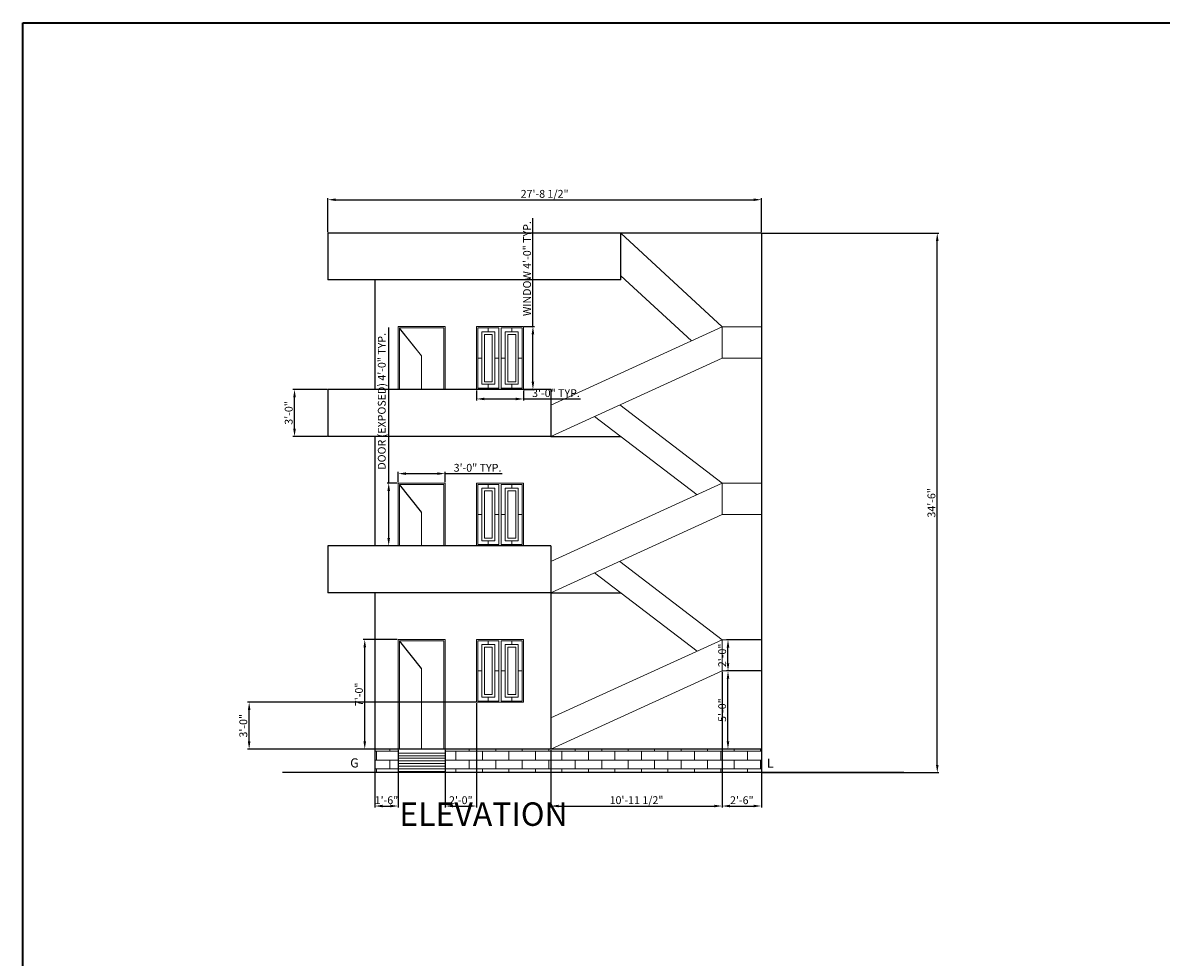
# Model space of a CAD drawing. Units: millimetres. Extents: x 50579 to 52843, y 62224 to 63803.
# Tile 2 of 5: x 50579 to 51453, y 63086 to 63803. Entities that reach past the tile are written whole.
import ezdxf

# ---------------------------------------------------------------- set-up
doc = ezdxf.new("R2010")
doc.units = ezdxf.units.MM
for name, color, linetype, lineweight in [('A-ANNO-DIMS', 2, 'Continuous', 18), ('A-ANNO-SYMB', 6, 'Continuous', 18), ('A-ANNO-TITL', 4, 'Continuous', 25), ('A-ANNO-TTLB', 7, 'Continuous', 35), ('A-ELEV', 7, 'Continuous', 25), ('A-ELEV-OPEN', 7, 'Continuous', 18), ('A-ELEV-PATT', 8, 'Continuous', 13), ('A-ELEV-STRS', 7, 'Continuous', 18)]:
    doc.layers.add(name, color=color, linetype=linetype, lineweight=lineweight)
doc.styles.get("Standard").update_dxf_attribs({"font": 'arial.ttf'})
doc.dimstyles.new('ISO-25', dxfattribs={"dimtxt": 6, "dimasz": 6, "dimexe": 1.25, "dimexo": 0.625, "dimtad": 1, "dimdec": 0, "dimlunit": 3, "dimtxsty": 'Standard', "dimcen": 2.5, "dimadec": 0, "dimazin": 0, "dimtfac": 1, "dimtdec": 0, "dimtmove": 0, "dimatfit": 3, "dimfxl": 1, "dimarcsym": 0})

# ---------------------------------------------------------------- blocks, each defined once
blk = doc.blocks.new('DOOR-BALCONY-ELEV')
for p, q in [((36, 48.21), (0, 48.21)), ((0, 48.21), (0, 0)), ((35, 47.21), (1, 47.21)), ((1, 47.21), (1, 0)), ((1, 47.12), (18.01, 25.89)), ((1, 46.8), (17.9, 25.71)), ((35, 0), (35, 47.21)), ((36, 0), (36, 48.21)), ((17.9, 25.71), (17.9, 0)), ((18.01, 25.89), (18.01, 0)), ((0, 0), (36, 0))]:
    blk.add_line(p, q)
blk = doc.blocks.new('WIN-PAIRED-ELEV')
for p, q in [((9, 44.24), (9, 47.24)), ((14, 44.24), (14, 4)), ((17, 47.24), (17, 1)), ((19, 47.24), (19, 1)), ((22, 44.24), (22, 4)), ((27, 44.24), (27, 47.24)), ((4, 24.12), (1, 24.12)), ((17, 24.12), (14, 24.12)), ((19, 24.12), (22, 24.12)), ((32, 24.12), (35, 24.12)), ((9, 4), (9, 1)), ((27, 4), (27, 1))]:
    blk.add_line(p, q)
for points in [[(0, 48.24), (36, 48.24), (36, 0), (0, 0)], [(12, 6), (6, 6), (6, 42.24), (12, 42.24)], [(24, 42.24), (30, 42.24), (30, 6), (24, 6)]]:
    blk.add_lwpolyline(points, close=True)
for points in [[(17, 1), (1, 1), (1, 47.24), (17, 47.24)], [(14, 4), (4, 4), (4, 44.24), (14, 44.24)], [(19, 47.24), (35, 47.24), (35, 1), (19, 1)], [(22, 44.24), (32, 44.24), (32, 4), (22, 4)]]:
    blk.add_lwpolyline(points)
blk = doc.blocks.new('*D37')
at = {"layer": 'A-ANNO-DIMS', "color": 0, "lineweight": -2, "transparency": 16777216}
for p, q in [((50860.17, 63449.49), (50860.17, 63568.92)), ((50866.77, 63449.49), (50858.92, 63449.49)), ((50860.17, 63407.28), (50860.17, 63443.49)), ((50866.77, 63401.28), (50858.92, 63401.28))]:
    blk.add_line(p, q, dxfattribs=at)
at = {"layer": 'A-ANNO-DIMS', "color": 0, "transparency": 16777216}
for points in [[(50859.17, 63443.49), (50861.17, 63443.49), (50860.17, 63449.49)], [(50859.17, 63407.28), (50861.17, 63407.28), (50860.17, 63401.28)]]:
    blk.add_solid(points, dxfattribs=at)
at = {"layer": 'Defpoints', "color": 0, "transparency": 16777216}
for p in [(50860.17, 63449.49), (50867.4, 63449.49), (50867.4, 63401.28)]:
    blk.add_point(p, dxfattribs=at)
at = {"layer": 'A-ANNO-DIMS', "color": 0, "transparency": 16777216, "insert": (50855.61, 63512.2), "char_height": 6, "attachment_point": 5, "rotation": 90}
blk.add_mtext('DOOR (EXPOSED) 4\'-0" TYP.', dxfattribs=at)
blk = doc.blocks.new('*D38')
at = {"layer": 'A-ANNO-DIMS', "color": 0, "lineweight": -2, "transparency": 16777216}
for p, q in [((50867.4, 63450.11), (50867.4, 63457.97)), ((50873.4, 63456.72), (50897.4, 63456.72)), ((50903.4, 63450.11), (50903.4, 63457.97)), ((50903.4, 63456.72), (50947.22, 63456.72))]:
    blk.add_line(p, q, dxfattribs=at)
at = {"layer": 'A-ANNO-DIMS', "color": 0, "transparency": 16777216}
for points in [[(50873.4, 63457.72), (50873.4, 63455.72), (50867.4, 63456.72)], [(50897.4, 63457.72), (50897.4, 63455.72), (50903.4, 63456.72)]]:
    blk.add_solid(points, dxfattribs=at)
at = {"layer": 'Defpoints', "color": 0, "transparency": 16777216}
for p in [(50903.4, 63456.72), (50867.4, 63449.49), (50903.4, 63449.49)]:
    blk.add_point(p, dxfattribs=at)
at = {"layer": 'A-ANNO-DIMS', "color": 0, "transparency": 16777216, "insert": (50928.31, 63460.41), "char_height": 6, "attachment_point": 5}
blk.add_mtext('3\'-0" TYP.', dxfattribs=at)
blk = doc.blocks.new('*D39')
at = {"layer": 'A-ANNO-DIMS', "color": 0, "lineweight": -2, "transparency": 16777216}
for p, q in [((50970.79, 63569.49), (50970.79, 63652.66)), ((50964.18, 63569.49), (50972.04, 63569.49)), ((50970.79, 63527.25), (50970.79, 63563.49)), ((50964.18, 63521.25), (50972.04, 63521.25))]:
    blk.add_line(p, q, dxfattribs=at)
at = {"layer": 'A-ANNO-DIMS', "color": 0, "transparency": 16777216}
for points in [[(50969.79, 63563.49), (50971.79, 63563.49), (50970.79, 63569.49)], [(50969.79, 63527.25), (50971.79, 63527.25), (50970.79, 63521.25)]]:
    blk.add_solid(points, dxfattribs=at)
at = {"layer": 'Defpoints', "color": 0, "transparency": 16777216}
for p in [(50963.56, 63569.49), (50970.79, 63569.49), (50963.56, 63521.25)]:
    blk.add_point(p, dxfattribs=at)
at = {"layer": 'A-ANNO-DIMS', "color": 0, "transparency": 16777216, "insert": (50967.06, 63614.07), "char_height": 6, "attachment_point": 5, "rotation": 90}
blk.add_mtext('WINDOW 4\'-0" TYP.', dxfattribs=at)
blk = doc.blocks.new('*D40')
at = {"layer": 'A-ANNO-DIMS', "color": 0, "lineweight": -2, "transparency": 16777216}
for p, q in [((50927.56, 63520.62), (50927.56, 63512.76)), ((50963.56, 63520.62), (50963.56, 63512.76)), ((50933.56, 63514.01), (50957.56, 63514.01)), ((50963.56, 63514.01), (51007.37, 63514.01))]:
    blk.add_line(p, q, dxfattribs=at)
at = {"layer": 'A-ANNO-DIMS', "color": 0, "transparency": 16777216}
for points in [[(50933.56, 63515.01), (50933.56, 63513.01), (50927.56, 63514.01)], [(50957.56, 63515.01), (50957.56, 63513.01), (50963.56, 63514.01)]]:
    blk.add_solid(points, dxfattribs=at)
at = {"layer": 'Defpoints', "color": 0, "transparency": 16777216}
for p in [(50927.56, 63521.25), (50963.56, 63521.25), (50963.56, 63514.01)]:
    blk.add_point(p, dxfattribs=at)
at = {"layer": 'A-ANNO-DIMS', "color": 0, "transparency": 16777216, "insert": (50988.47, 63517.7), "char_height": 6, "attachment_point": 5}
blk.add_mtext('3\'-0" TYP.', dxfattribs=at)
blk = doc.blocks.new('*D45')
at = {"layer": 'A-ANNO-DIMS', "color": 0, "lineweight": -2, "transparency": 16777216}
for p, q in [((50813.52, 63641.9), (50813.52, 63668.13)), ((50819.52, 63666.88), (51140.02, 63666.88)), ((51146.02, 63641.9), (51146.02, 63668.13))]:
    blk.add_line(p, q, dxfattribs=at)
at = {"layer": 'A-ANNO-DIMS', "color": 0, "transparency": 16777216}
for points in [[(50819.52, 63667.88), (50819.52, 63665.88), (50813.52, 63666.88)], [(51140.02, 63667.88), (51140.02, 63665.88), (51146.02, 63666.88)]]:
    blk.add_solid(points, dxfattribs=at)
at = {"layer": 'Defpoints', "color": 0, "transparency": 16777216}
for p in [(51146.02, 63666.88), (50813.52, 63641.28), (51146.02, 63641.28)]:
    blk.add_point(p, dxfattribs=at)
at = {"layer": 'A-ANNO-DIMS', "color": 0, "transparency": 16777216, "insert": (50979.77, 63670.61), "char_height": 6, "attachment_point": 5}
blk.add_mtext('27\'-8 1/2"', dxfattribs=at)
blk = doc.blocks.new('*D46')
at = {"layer": 'A-ANNO-DIMS', "color": 0, "lineweight": -2, "transparency": 16777216}
for p, q in [((51146.64, 63641.28), (51282.2, 63641.28)), ((51280.95, 63233.28), (51280.95, 63635.28)), ((51146.64, 63227.28), (51282.2, 63227.28))]:
    blk.add_line(p, q, dxfattribs=at)
at = {"layer": 'A-ANNO-DIMS', "color": 0, "transparency": 16777216}
for points in [[(51279.95, 63635.28), (51281.95, 63635.28), (51280.95, 63641.28)], [(51279.95, 63233.28), (51281.95, 63233.28), (51280.95, 63227.28)]]:
    blk.add_solid(points, dxfattribs=at)
at = {"layer": 'Defpoints', "color": 0, "transparency": 16777216}
for p in [(51146.02, 63641.28), (51280.95, 63641.28), (51146.02, 63227.28)]:
    blk.add_point(p, dxfattribs=at)
at = {"layer": 'A-ANNO-DIMS', "color": 0, "transparency": 16777216, "insert": (51277.26, 63434.28), "char_height": 6, "attachment_point": 5, "rotation": 90}
blk.add_mtext('34\'-6"', dxfattribs=at)
blk = doc.blocks.new('*D49')
at = {"layer": 'A-ANNO-DIMS', "color": 0, "lineweight": -2, "transparency": 16777216}
for p, q in [((50849.52, 63244.65), (50849.52, 63200.43)), ((50867.4, 63244.65), (50867.4, 63200.43)), ((50855.52, 63201.68), (50861.4, 63201.68))]:
    blk.add_line(p, q, dxfattribs=at)
at = {"layer": 'A-ANNO-DIMS', "color": 0, "transparency": 16777216}
for points in [[(50855.52, 63202.68), (50855.52, 63200.68), (50849.52, 63201.68)], [(50861.4, 63202.68), (50861.4, 63200.68), (50867.4, 63201.68)]]:
    blk.add_solid(points, dxfattribs=at)
at = {"layer": 'Defpoints', "color": 0, "transparency": 16777216}
for p in [(50849.52, 63245.28), (50867.4, 63245.28), (50867.4, 63201.68)]:
    blk.add_point(p, dxfattribs=at)
at = {"layer": 'A-ANNO-DIMS', "color": 0, "transparency": 16777216, "insert": (50858.46, 63205.37), "char_height": 6, "attachment_point": 5}
blk.add_mtext('1\'-6"', dxfattribs=at)
blk = doc.blocks.new('*D50')
at = {"layer": 'A-ANNO-DIMS', "color": 0, "lineweight": -2, "transparency": 16777216}
for p, q in [((50927.56, 63280.62), (50927.56, 63200.43)), ((50903.4, 63244.65), (50903.4, 63200.43)), ((50909.4, 63201.68), (50921.56, 63201.68))]:
    blk.add_line(p, q, dxfattribs=at)
at = {"layer": 'A-ANNO-DIMS', "color": 0, "transparency": 16777216}
for points in [[(50909.4, 63202.68), (50909.4, 63200.68), (50903.4, 63201.68)], [(50921.56, 63202.68), (50921.56, 63200.68), (50927.56, 63201.68)]]:
    blk.add_solid(points, dxfattribs=at)
at = {"layer": 'Defpoints', "color": 0, "transparency": 16777216}
for p in [(50927.56, 63281.25), (50903.4, 63245.28), (50927.56, 63201.68)]:
    blk.add_point(p, dxfattribs=at)
at = {"layer": 'A-ANNO-DIMS', "color": 0, "transparency": 16777216, "insert": (50915.48, 63205.37), "char_height": 6, "attachment_point": 5}
blk.add_mtext('2\'-0"', dxfattribs=at)
blk = doc.blocks.new('*D51')
at = {"layer": 'A-ANNO-DIMS', "color": 0, "lineweight": -2, "transparency": 16777216}
for p, q in [((51116.02, 63304.65), (51116.02, 63200.43)), ((50984.52, 63244.65), (50984.52, 63200.43)), ((50990.52, 63201.68), (51110.02, 63201.68))]:
    blk.add_line(p, q, dxfattribs=at)
at = {"layer": 'A-ANNO-DIMS', "color": 0, "transparency": 16777216}
for points in [[(50990.52, 63202.68), (50990.52, 63200.68), (50984.52, 63201.68)], [(51110.02, 63202.68), (51110.02, 63200.68), (51116.02, 63201.68)]]:
    blk.add_solid(points, dxfattribs=at)
at = {"layer": 'Defpoints', "color": 0, "transparency": 16777216}
for p in [(51116.02, 63305.28), (50984.52, 63245.28), (51116.02, 63201.68)]:
    blk.add_point(p, dxfattribs=at)
at = {"layer": 'A-ANNO-DIMS', "color": 0, "transparency": 16777216, "insert": (51050.27, 63205.41), "char_height": 6, "attachment_point": 5}
blk.add_mtext('10\'-11 1/2"', dxfattribs=at)
blk = doc.blocks.new('*D52')
at = {"layer": 'A-ANNO-DIMS', "color": 0, "lineweight": -2, "transparency": 16777216}
for p, q in [((51116.02, 63304.65), (51116.02, 63200.43)), ((51146.02, 63244.65), (51146.02, 63200.43)), ((51122.02, 63201.68), (51140.02, 63201.68))]:
    blk.add_line(p, q, dxfattribs=at)
at = {"layer": 'A-ANNO-DIMS', "color": 0, "transparency": 16777216}
for points in [[(51122.02, 63202.68), (51122.02, 63200.68), (51116.02, 63201.68)], [(51140.02, 63202.68), (51140.02, 63200.68), (51146.02, 63201.68)]]:
    blk.add_solid(points, dxfattribs=at)
at = {"layer": 'Defpoints', "color": 0, "transparency": 16777216}
for p in [(51116.02, 63305.28), (51146.02, 63245.28), (51146.02, 63201.68)]:
    blk.add_point(p, dxfattribs=at)
at = {"layer": 'A-ANNO-DIMS', "color": 0, "transparency": 16777216, "insert": (51131.02, 63205.37), "char_height": 6, "attachment_point": 5}
blk.add_mtext('2\'-6"', dxfattribs=at)
blk = doc.blocks.new('*D53')
at = {"layer": 'A-ANNO-DIMS', "color": 0, "lineweight": -2, "transparency": 16777216}
for p, q in [((50926.93, 63281.25), (50751.87, 63281.25)), ((50753.12, 63251.28), (50753.12, 63275.25)), ((50866.77, 63245.28), (50751.87, 63245.28))]:
    blk.add_line(p, q, dxfattribs=at)
at = {"layer": 'A-ANNO-DIMS', "color": 0, "transparency": 16777216}
for points in [[(50752.12, 63275.25), (50754.12, 63275.25), (50753.12, 63281.25)], [(50752.12, 63251.28), (50754.12, 63251.28), (50753.12, 63245.28)]]:
    blk.add_solid(points, dxfattribs=at)
at = {"layer": 'Defpoints', "color": 0, "transparency": 16777216}
for p in [(50753.12, 63281.25), (50927.56, 63281.25), (50867.4, 63245.28)]:
    blk.add_point(p, dxfattribs=at)
at = {"layer": 'A-ANNO-DIMS', "color": 0, "transparency": 16777216, "insert": (50749.42, 63263.26), "char_height": 6, "attachment_point": 5, "rotation": 90}
blk.add_mtext('3\'-0"', dxfattribs=at)
blk = doc.blocks.new('*D54')
at = {"layer": 'A-ANNO-DIMS', "color": 0, "lineweight": -2, "transparency": 16777216}
for p, q in [((50866.77, 63329.49), (50840.55, 63329.49)), ((50841.8, 63251.28), (50841.8, 63323.49)), ((50866.77, 63245.28), (50840.55, 63245.28))]:
    blk.add_line(p, q, dxfattribs=at)
at = {"layer": 'A-ANNO-DIMS', "color": 0, "transparency": 16777216}
for points in [[(50840.8, 63323.49), (50842.8, 63323.49), (50841.8, 63329.49)], [(50840.8, 63251.28), (50842.8, 63251.28), (50841.8, 63245.28)]]:
    blk.add_solid(points, dxfattribs=at)
at = {"layer": 'Defpoints', "color": 0, "transparency": 16777216}
for p in [(50841.8, 63329.49), (50867.4, 63329.49), (50867.4, 63245.28)]:
    blk.add_point(p, dxfattribs=at)
at = {"layer": 'A-ANNO-DIMS', "color": 0, "transparency": 16777216, "insert": (50838.11, 63287.38), "char_height": 6, "attachment_point": 5, "rotation": 90}
blk.add_mtext('7\'-0"', dxfattribs=at)
blk = doc.blocks.new('*D55')
at = {"layer": 'A-ANNO-DIMS', "color": 0, "lineweight": -2, "transparency": 16777216}
for p, q in [((51145.39, 63305.28), (51119.17, 63305.28)), ((51120.42, 63251.28), (51120.42, 63299.28)), ((51145.39, 63245.28), (51119.17, 63245.28))]:
    blk.add_line(p, q, dxfattribs=at)
at = {"layer": 'A-ANNO-DIMS', "color": 0, "transparency": 16777216}
for points in [[(51119.42, 63299.28), (51121.42, 63299.28), (51120.42, 63305.28)], [(51119.42, 63251.28), (51121.42, 63251.28), (51120.42, 63245.28)]]:
    blk.add_solid(points, dxfattribs=at)
at = {"layer": 'Defpoints', "color": 0, "transparency": 16777216}
for p in [(51120.42, 63305.28), (51146.02, 63305.28), (51146.02, 63245.28)]:
    blk.add_point(p, dxfattribs=at)
at = {"layer": 'A-ANNO-DIMS', "color": 0, "transparency": 16777216, "insert": (51116.73, 63275.28), "char_height": 6, "attachment_point": 5, "rotation": 90}
blk.add_mtext('5\'-0"', dxfattribs=at)
blk = doc.blocks.new('*D56')
at = {"layer": 'A-ANNO-DIMS', "color": 0, "lineweight": -2, "transparency": 16777216}
for p, q in [((51145.39, 63329.28), (51119.17, 63329.28)), ((51120.42, 63311.28), (51120.42, 63323.28)), ((51145.39, 63305.28), (51119.17, 63305.28))]:
    blk.add_line(p, q, dxfattribs=at)
at = {"layer": 'A-ANNO-DIMS', "color": 0, "transparency": 16777216}
for points in [[(51119.42, 63323.28), (51121.42, 63323.28), (51120.42, 63329.28)], [(51119.42, 63311.28), (51121.42, 63311.28), (51120.42, 63305.28)]]:
    blk.add_solid(points, dxfattribs=at)
at = {"layer": 'Defpoints', "color": 0, "transparency": 16777216}
for p in [(51120.42, 63329.28), (51146.02, 63329.28), (51146.02, 63305.28)]:
    blk.add_point(p, dxfattribs=at)
at = {"layer": 'A-ANNO-DIMS', "color": 0, "transparency": 16777216, "insert": (51116.73, 63317.28), "char_height": 6, "attachment_point": 5, "rotation": 90}
blk.add_mtext('2\'-0"', dxfattribs=at)
blk = doc.blocks.new('*D57')
at = {"layer": 'A-ANNO-DIMS', "color": 0, "lineweight": -2, "transparency": 16777216}
for p, q in [((50812.89, 63521.28), (50786.67, 63521.28)), ((50787.92, 63491.28), (50787.92, 63515.28)), ((50812.89, 63485.28), (50786.67, 63485.28))]:
    blk.add_line(p, q, dxfattribs=at)
at = {"layer": 'A-ANNO-DIMS', "color": 0, "transparency": 16777216}
for points in [[(50786.92, 63515.28), (50788.92, 63515.28), (50787.92, 63521.28)], [(50786.92, 63491.28), (50788.92, 63491.28), (50787.92, 63485.28)]]:
    blk.add_solid(points, dxfattribs=at)
at = {"layer": 'Defpoints', "color": 0, "transparency": 16777216}
for p in [(50787.92, 63521.28), (50813.52, 63521.28), (50813.52, 63485.28)]:
    blk.add_point(p, dxfattribs=at)
at = {"layer": 'A-ANNO-DIMS', "color": 0, "transparency": 16777216, "insert": (50784.23, 63503.28), "char_height": 6, "attachment_point": 5, "rotation": 90}
blk.add_mtext('3\'-0"', dxfattribs=at)

msp = doc.modelspace()

# ---------------------------------------------------------------- hatches: boundary and pattern name
at = {"layer": 'A-ELEV-PATT'}
h = msp.add_hatch(dxfattribs=at)
h.set_pattern_fill('AR-BRSTD', color=256, scale=0.1)
h.paths.add_polyline_path([(50867.4, 63245.28), (50849.52, 63245.28), (50849.52, 63227.28), (50867.4, 63227.28)])
h = msp.add_hatch(dxfattribs=at)
h.set_pattern_fill('AR-BRSTD', color=256, scale=0.1)
h.paths.add_polyline_path([(51146.02, 63245.28), (50903.4, 63245.28), (50903.4, 63227.28), (51146.02, 63227.28)])

# ---------------------------------------------------------------- linework, layer by layer
at = {"layer": 'A-ANNO-TTLB'}
msp.add_lwpolyline([(50579.46, 63802.65), (52843.1, 63802.65), (52843.1, 62224.04), (50579.46, 62224.04)], close=True, dxfattribs=at)
at = {"layer": 'A-ELEV'}
for p, q in [((51146.02, 63641.28), (50813.52, 63641.28)), ((50813.52, 63641.28), (50813.52, 63605.28)), ((51038.17, 63605.28), (51038.17, 63641.28)), ((51146.02, 63641.28), (51146.02, 63227.28)), ((51038.17, 63605.28), (50813.52, 63605.28)), ((50849.52, 63605.28), (50849.52, 63521.28)), ((50984.52, 63521.28), (50813.52, 63521.28)), ((50813.52, 63521.28), (50813.52, 63485.28)), ((50984.52, 63521.28), (50984.52, 63485.28)), ((50984.52, 63485.28), (50813.52, 63485.28)), ((50849.52, 63485.28), (50849.52, 63401.28)), ((50984.52, 63485.28), (51038.17, 63485.28)), ((50813.52, 63401.28), (50813.52, 63365.28)), ((50984.52, 63401.28), (50813.52, 63401.28)), ((50984.52, 63401.28), (50984.52, 63245.28)), ((50984.52, 63365.28), (50813.52, 63365.28)), ((50849.52, 63365.28), (50849.52, 63227.28)), ((50984.52, 63365.28), (51038.17, 63365.28)), ((51146.02, 63245.28), (50849.52, 63245.28)), ((51255.35, 63227.28), (50778.72, 63227.28))]:
    msp.add_line(p, q, dxfattribs=at)
at = {"layer": 'A-ELEV-OPEN'}
for p, q in [((50868.4, 63328.4), (50885.41, 63307.17)), ((50868.4, 63328.08), (50885.3, 63306.99)), ((50936.56, 63325.49), (50936.56, 63328.49)), ((50944.56, 63328.49), (50944.56, 63282.25)), ((50946.56, 63328.49), (50946.56, 63282.25)), ((50954.56, 63325.49), (50954.56, 63328.49)), ((50885.3, 63306.99), (50885.3, 63245.28)), ((50885.41, 63307.17), (50885.41, 63245.28)), ((50931.56, 63305.37), (50928.56, 63305.37)), ((50944.56, 63305.37), (50941.56, 63305.37)), ((50946.56, 63305.37), (50949.56, 63305.37)), ((50959.56, 63305.37), (50962.56, 63305.37)), ((50936.56, 63285.25), (50936.56, 63282.25)), ((50954.56, 63285.25), (50954.56, 63282.25))]:
    msp.add_line(p, q, dxfattribs=at)
for points in [[(50867.4, 63245.28), (50903.4, 63245.28), (50903.4, 63329.49), (50867.4, 63329.49)], [(50927.56, 63329.49), (50963.56, 63329.49), (50963.56, 63281.25), (50927.56, 63281.25)], [(50941.56, 63285.25), (50931.56, 63285.25), (50931.56, 63325.49), (50941.56, 63325.49)], [(50939.56, 63287.25), (50933.56, 63287.25), (50933.56, 63323.49), (50939.56, 63323.49)], [(50949.56, 63325.49), (50959.56, 63325.49), (50959.56, 63285.25), (50949.56, 63285.25)], [(50951.56, 63323.49), (50957.56, 63323.49), (50957.56, 63287.25), (50951.56, 63287.25)]]:
    msp.add_lwpolyline(points, close=True, dxfattribs=at)
for points in [[(50902.4, 63245.28), (50902.4, 63328.49), (50868.4, 63328.49), (50868.4, 63245.28)], [(50944.56, 63282.25), (50928.56, 63282.25), (50928.56, 63328.49), (50944.56, 63328.49)], [(50946.56, 63328.49), (50962.56, 63328.49), (50962.56, 63282.25), (50946.56, 63282.25)], [(50885.3, 63246.28), (50885.41, 63246.28)]]:
    msp.add_lwpolyline(points, dxfattribs=at)
at = {"layer": 'A-ELEV-STRS'}
for p, q in [((51038.17, 63641.28), (51116.02, 63569.28)), ((51038.17, 63608.59), (51092.35, 63558.48)), ((50984.52, 63509.28), (51116.02, 63569.28)), ((51116.02, 63569.28), (51116.02, 63545.28)), ((51146.02, 63569.28), (51116.02, 63569.28)), ((50984.52, 63485.28), (51116.02, 63545.28)), ((51146.02, 63545.28), (51116.02, 63545.28)), ((51116.02, 63449.28), (51037.38, 63509.4)), ((51096.75, 63440.49), (51018.12, 63500.61)), ((50984.52, 63389.28), (51116.02, 63449.28)), ((51146.02, 63449.28), (51116.02, 63449.28)), ((51116.02, 63449.28), (51116.02, 63425.28)), ((50984.52, 63365.28), (51116.02, 63425.28)), ((51146.02, 63425.28), (51116.02, 63425.28)), ((51116.02, 63329.28), (51037.38, 63389.4)), ((51096.75, 63320.49), (51018.12, 63380.61)), ((50984.52, 63269.28), (51116.02, 63329.28)), ((51146.02, 63329.28), (51116.02, 63329.28)), ((51116.02, 63329.28), (51116.02, 63305.28)), ((50984.52, 63245.28), (51116.02, 63305.28)), ((51146.02, 63305.28), (51116.02, 63305.28)), ((50867.4, 63245.28), (50867.4, 63227.28)), ((50903.4, 63245.28), (50903.4, 63227.28)), ((50867.4, 63242.28), (50903.4, 63242.28)), ((50867.4, 63240.28), (50903.4, 63240.28)), ((50867.4, 63238.28), (50903.4, 63238.28)), ((50867.4, 63236.28), (50903.4, 63236.28)), ((50867.4, 63234.28), (50903.4, 63234.28)), ((50867.4, 63232.28), (50903.4, 63232.28)), ((50867.4, 63230.28), (50903.4, 63230.28)), ((50867.4, 63228.28), (50903.4, 63228.28))]:
    msp.add_line(p, q, dxfattribs=at)

# ---------------------------------------------------------------- block references
at = {"layer": 'A-ELEV-OPEN'}
for name, p in [('DOOR-BALCONY-ELEV', (50867.4, 63521.28)), ('WIN-PAIRED-ELEV', (50927.56, 63521.25)), ('DOOR-BALCONY-ELEV', (50867.4, 63401.28)), ('WIN-PAIRED-ELEV', (50927.56, 63401.25))]:
    msp.add_blockref(name, p, dxfattribs=at)

# ---------------------------------------------------------------- texts
at = {"layer": 'A-ANNO-SYMB', "char_height": 7, "attachment_point": 1}
for s, insert in [('  G', (50826.33, 63238.26)), ('  L', (51145.99, 63238.04))]:
    msp.add_mtext_dynamic_manual_height_columns(s, width=13.8936, gutter_width=12.5, heights=[0], dxfattribs=dict(at, insert=insert))
at = {"layer": 'A-ANNO-TITL', "insert": (50857.28, 63204.47), "char_height": 18, "attachment_point": 1}
msp.add_mtext_dynamic_manual_height_columns('  ELEVATION', width=341.9217, gutter_width=12.5, heights=[0], dxfattribs=at)

# ---------------------------------------------------------------- dimensions: what is measured, and where the dimension line sits
at = {"layer": 'A-ANNO-DIMS'}
for base, p1, p2, picture, middle in [((51146.02, 63666.88), (50813.52, 63641.28), (51146.02, 63641.28), '*D45', (50979.77, 63670.61)), ((51116.02, 63201.68), (50984.52, 63245.28), (51116.02, 63305.28), '*D51', (51050.27, 63205.41)), ((51146.02, 63201.68), (51116.02, 63305.28), (51146.02, 63245.28), '*D52', (51131.02, 63205.37)), ((50927.56, 63201.68), (50903.4, 63245.28), (50927.56, 63281.25), '*D50', (50915.48, 63205.37)), ((50867.4, 63201.68), (50849.52, 63245.28), (50867.4, 63245.28), '*D49', (50858.46, 63205.37))]:
    dim = msp.add_linear_dim(base=base, p1=p1, p2=p2, dimstyle='ISO-25', override={"dimdec": 1, "dimlfac": 1, "dimrnd": 0, "dimzin": 1, "dimdsep": 46, "dimlunit": 4, "dimfrac": 2}, dxfattribs=at)
    dim.commit()
    dim.dimension.update_dxf_attribs({"geometry": picture, "text_midpoint": middle})
for base, p1, p2, text, picture, middle in [((50970.79, 63569.49), (50963.56, 63521.25), (50963.56, 63569.49), 'WINDOW <> TYP.', '*D39', (50967.06, 63614.07)), ((50860.17, 63449.49), (50867.4, 63401.28), (50867.4, 63449.49), 'DOOR (EXPOSED) <> TYP.', '*D37', (50855.61, 63512.2))]:
    dim = msp.add_linear_dim(base=base, p1=p1, p2=p2, angle=90, text=text, dimstyle='ISO-25', override={"dimdec": 1, "dimlfac": 1, "dimrnd": 0, "dimzin": 1, "dimdsep": 46, "dimlunit": 4, "dimfrac": 2}, dxfattribs=at)
    dim.commit()
    dim.dimension.update_dxf_attribs({"geometry": picture, "text_midpoint": middle})
for base, p1, p2, picture, middle in [((51280.95, 63641.28), (51146.02, 63227.28), (51146.02, 63641.28), '*D46', (51277.26, 63434.28)), ((50787.92, 63521.28), (50813.52, 63485.28), (50813.52, 63521.28), '*D57', (50784.23, 63503.28)), ((50841.8, 63329.49), (50867.4, 63245.28), (50867.4, 63329.49), '*D54', (50838.11, 63287.38)), ((51120.42, 63329.28), (51146.02, 63305.28), (51146.02, 63329.28), '*D56', (51116.73, 63317.28)), ((51120.42, 63305.28), (51146.02, 63245.28), (51146.02, 63305.28), '*D55', (51116.73, 63275.28)), ((50753.12, 63281.25), (50867.4, 63245.28), (50927.56, 63281.25), '*D53', (50749.42, 63263.26))]:
    dim = msp.add_linear_dim(base=base, p1=p1, p2=p2, angle=90, dimstyle='ISO-25', override={"dimdec": 1, "dimlfac": 1, "dimrnd": 0, "dimzin": 1, "dimdsep": 46, "dimlunit": 4, "dimfrac": 2}, dxfattribs=at)
    dim.commit()
    dim.dimension.update_dxf_attribs({"geometry": picture, "text_midpoint": middle})
for base, p1, p2, picture, middle in [((50963.56, 63514.01), (50927.56, 63521.25), (50963.56, 63521.25), '*D40', (50988.47, 63517.7)), ((50903.4, 63456.72), (50867.4, 63449.49), (50903.4, 63449.49), '*D38', (50928.31, 63460.41))]:
    dim = msp.add_linear_dim(base=base, p1=p1, p2=p2, text='<> TYP.', dimstyle='ISO-25', override={"dimdec": 1, "dimlfac": 1, "dimrnd": 0, "dimzin": 1, "dimdsep": 46, "dimlunit": 4, "dimfrac": 2}, dxfattribs=at)
    dim.commit()
    dim.dimension.update_dxf_attribs({"geometry": picture, "text_midpoint": middle})

doc.saveas('drawing.dxf')
